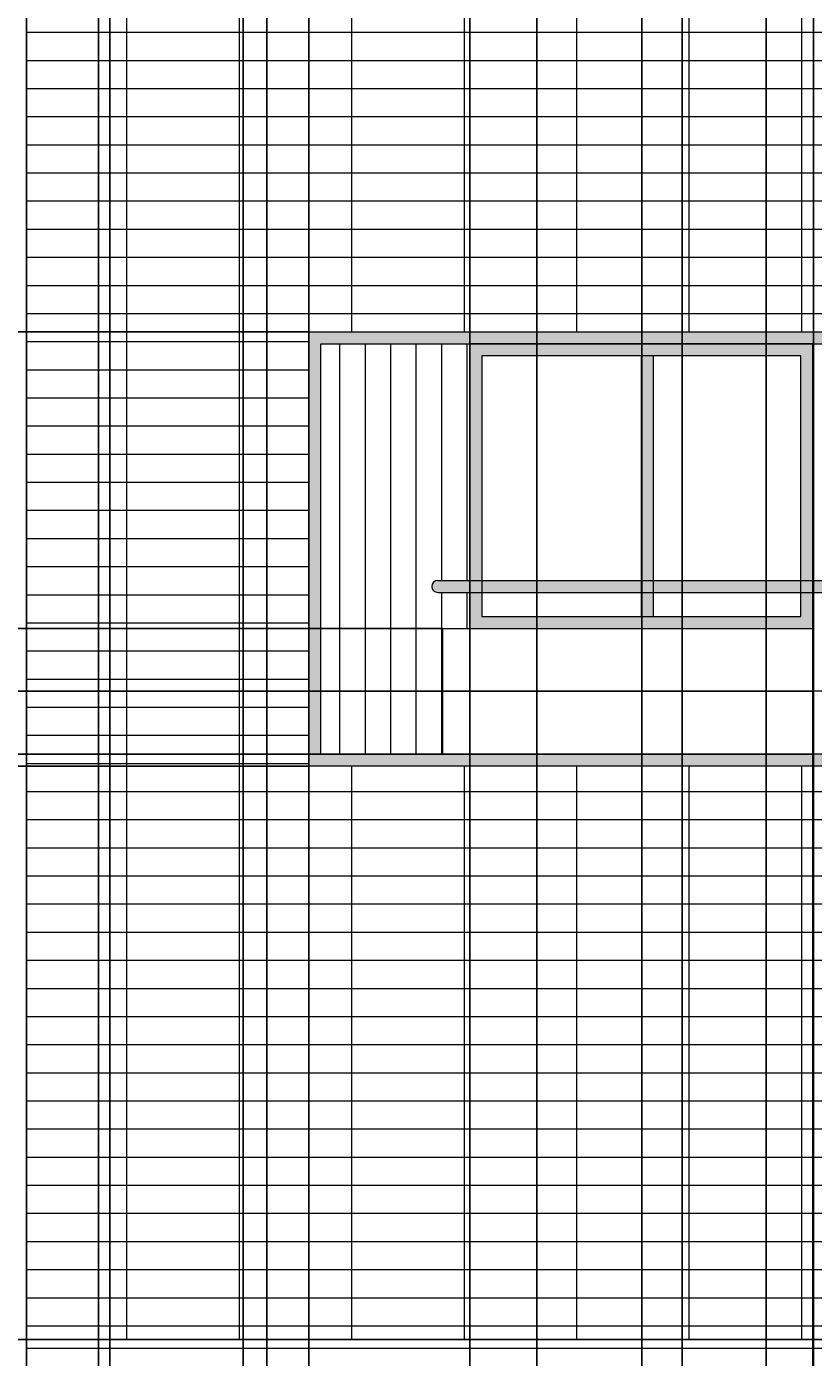
# Model space of a CAD drawing. Units: inches. Extents: x 241 to 943, y 109 to 1396.
# Tile 7 of 34: x 377 to 508, y 398 to 620. Entities that reach past the tile are written whole.
import ezdxf

# ---------------------------------------------------------------- set-up
doc = ezdxf.new("R2010")
doc.units = ezdxf.units.IN
doc.header["$MEASUREMENT"] = 0
for name, color, linetype, lineweight in [('A-ANNO-DIMS', 2, 'Continuous', 18), ('A-ELEV', 7, 'Continuous', 25), ('A-ELEV-SHAD', 9, 'Continuous', 13), ('A-GLAZ', 4, 'Continuous', 18), ('A-GLAZ-PATT', 18, 'Continuous', 13), ('A-WALL-PATT', 8, 'Continuous', 13)]:
    doc.layers.add(name, color=color, linetype=linetype, lineweight=lineweight)
doc.styles.get("Standard").update_dxf_attribs({"font": 'arial.ttf'})
doc.dimstyles.get("Standard").update_dxf_attribs({"dimtxt": 1.4375, "dimasz": 0.18, "dimexe": 0.18, "dimexo": 0.0625, "dimgap": 0.09, "dimtad": 0, "dimtih": 1, "dimtoh": 1, "dimdec": 4, "dimzin": 0, "dimdsep": 46, "dimlunit": 4, "dimtxsty": 'Standard', "dimcen": 0.09, "dimadec": 0, "dimazin": 0, "dimtfac": 1, "dimtdec": 4, "dimtofl": 0, "dimtmove": 0, "dimatfit": 3, "dimfxl": 1, "dimtolj": 1, "dimtzin": 0, "dimarcsym": 0})

# ---------------------------------------------------------------- blocks, each defined once
blk = doc.blocks.new('*D7')
at = {"layer": 'A-ANNO-DIMS', "color": 0, "lineweight": -2, "transparency": 16777216}
for p, q in [((508.24, 1336.12), (244.31, 1336.12)), ((244.49, 1335.94), (244.49, 753.25)), ((244.49, 168.92), (244.49, 751.6)), ((303.17, 168.74), (244.31, 168.74))]:
    blk.add_line(p, q, dxfattribs=at)
at = {"layer": 'A-ANNO-DIMS', "color": 0, "transparency": 16777216}
for points in [[(244.46, 1335.94), (244.52, 1335.94), (244.49, 1336.12)], [(244.46, 168.92), (244.52, 168.92), (244.49, 168.74)]]:
    blk.add_solid(points, dxfattribs=at)
at = {"layer": 'Defpoints', "color": 0, "transparency": 16777216}
for p in [(244.49, 1336.12), (508.31, 1336.12), (303.24, 168.74)]:
    blk.add_point(p, dxfattribs=at)
at = {"layer": 'A-ANNO-DIMS', "color": 0, "transparency": 16777216, "insert": (244.49, 752.43), "char_height": 1.438, "attachment_point": 5}
blk.add_mtext('\\A1;1167.4', dxfattribs=at)
blk = doc.blocks.new('*D8')
at = {"layer": 'A-ANNO-DIMS', "color": 0, "lineweight": -2, "transparency": 16777216}
for p, q in [((377.04, 396.94), (377.04, 1395.05)), ((377.22, 1394.87), (380.96, 1394.87)), ((390.71, 1394.87), (386.97, 1394.87)), ((390.89, 384.24), (390.89, 1395.05))]:
    blk.add_line(p, q, dxfattribs=at)
at = {"layer": 'A-ANNO-DIMS', "color": 0, "transparency": 16777216}
for points in [[(377.22, 1394.9), (377.22, 1394.84), (377.04, 1394.87)], [(390.71, 1394.9), (390.71, 1394.84), (390.89, 1394.87)]]:
    blk.add_solid(points, dxfattribs=at)
at = {"layer": 'Defpoints', "color": 0, "transparency": 16777216}
for p in [(390.89, 1394.87), (377.04, 396.88), (390.89, 384.18)]:
    blk.add_point(p, dxfattribs=at)
at = {"layer": 'A-ANNO-DIMS', "color": 0, "transparency": 16777216, "insert": (383.97, 1394.87), "char_height": 1.438, "attachment_point": 5}
blk.add_mtext('\\A1;13.856', dxfattribs=at)
blk = doc.blocks.new('*D9')
at = {"layer": 'A-ANNO-DIMS', "color": 0, "lineweight": -2, "transparency": 16777216}
for p, q in [((390.89, 384.24), (390.89, 1395.05)), ((391.07, 1394.87), (424.13, 1394.87)), ((461.93, 1394.87), (428.87, 1394.87)), ((462.11, 384.24), (462.11, 1395.05))]:
    blk.add_line(p, q, dxfattribs=at)
at = {"layer": 'A-ANNO-DIMS', "color": 0, "transparency": 16777216}
for points in [[(391.07, 1394.9), (391.07, 1394.84), (390.89, 1394.87)], [(461.93, 1394.9), (461.93, 1394.84), (462.11, 1394.87)]]:
    blk.add_solid(points, dxfattribs=at)
at = {"layer": 'Defpoints', "color": 0, "transparency": 16777216}
for p in [(462.11, 1394.87), (390.89, 384.18), (462.11, 384.18)]:
    blk.add_point(p, dxfattribs=at)
at = {"layer": 'A-ANNO-DIMS', "color": 0, "transparency": 16777216, "insert": (426.5, 1394.87), "char_height": 1.438, "attachment_point": 5}
blk.add_mtext('\\A1;71.21', dxfattribs=at)
blk = doc.blocks.new('*D10')
at = {"layer": 'A-ANNO-DIMS', "color": 0, "lineweight": -2, "transparency": 16777216}
for p, q in [((462.11, 384.24), (462.11, 1395.05)), ((462.29, 1394.87), (468.4, 1394.87)), ((479.42, 1394.87), (473.3, 1394.87)), ((479.6, 384.24), (479.6, 1395.05))]:
    blk.add_line(p, q, dxfattribs=at)
at = {"layer": 'A-ANNO-DIMS', "color": 0, "transparency": 16777216}
for points in [[(462.29, 1394.9), (462.29, 1394.84), (462.11, 1394.87)], [(479.42, 1394.9), (479.42, 1394.84), (479.6, 1394.87)]]:
    blk.add_solid(points, dxfattribs=at)
at = {"layer": 'Defpoints', "color": 0, "transparency": 16777216}
for p in [(479.6, 1394.87), (462.11, 384.18), (479.6, 384.18)]:
    blk.add_point(p, dxfattribs=at)
at = {"layer": 'A-ANNO-DIMS', "color": 0, "transparency": 16777216, "insert": (470.85, 1394.87), "char_height": 1.438, "attachment_point": 5}
blk.add_mtext('\\A1;17.49', dxfattribs=at)
blk = doc.blocks.new('*D11')
at = {"layer": 'A-ANNO-DIMS', "color": 0, "lineweight": -2, "transparency": 16777216}
for p, q in [((500.33, 384.24), (500.33, 1395.05)), ((500.51, 1394.87), (513.31, 1394.87)), ((530.05, 1394.87), (517.25, 1394.87)), ((530.23, 384.24), (530.23, 1395.05))]:
    blk.add_line(p, q, dxfattribs=at)
at = {"layer": 'A-ANNO-DIMS', "color": 0, "transparency": 16777216}
for points in [[(500.51, 1394.9), (500.51, 1394.84), (500.33, 1394.87)], [(530.05, 1394.9), (530.05, 1394.84), (530.23, 1394.87)]]:
    blk.add_solid(points, dxfattribs=at)
at = {"layer": 'Defpoints', "color": 0, "transparency": 16777216}
for p in [(530.23, 1394.87), (500.33, 384.18), (530.23, 384.18)]:
    blk.add_point(p, dxfattribs=at)
at = {"layer": 'A-ANNO-DIMS', "color": 0, "transparency": 16777216, "insert": (515.28, 1394.87), "char_height": 1.438, "attachment_point": 5}
blk.add_mtext('\\A1;29.9', dxfattribs=at)
blk = doc.blocks.new('*D32')
at = {"layer": 'A-ANNO-DIMS', "color": 0, "lineweight": -2, "transparency": 16777216}
for p, q in [((424.05, 568.83), (244.31, 568.83)), ((244.49, 568.65), (244.49, 533.46)), ((244.49, 496.62), (244.49, 531.81)), ((424.05, 496.44), (244.31, 496.44))]:
    blk.add_line(p, q, dxfattribs=at)
at = {"layer": 'A-ANNO-DIMS', "color": 0, "transparency": 16777216}
for points in [[(244.46, 568.65), (244.52, 568.65), (244.49, 568.83)], [(244.46, 496.62), (244.52, 496.62), (244.49, 496.44)]]:
    blk.add_solid(points, dxfattribs=at)
at = {"layer": 'Defpoints', "color": 0, "transparency": 16777216}
for p in [(244.49, 568.83), (424.11, 568.83), (424.11, 496.44)]:
    blk.add_point(p, dxfattribs=at)
at = {"layer": 'A-ANNO-DIMS', "color": 0, "transparency": 16777216, "insert": (244.49, 532.63), "char_height": 1.438, "attachment_point": 5}
blk.add_mtext('\\A1;72.39', dxfattribs=at)
blk = doc.blocks.new('*D33')
at = {"layer": 'A-ANNO-DIMS', "color": 0, "lineweight": -2, "transparency": 16777216}
for p, q in [((424.05, 628.4), (244.31, 628.4)), ((244.49, 628.22), (244.49, 599.44)), ((244.49, 569.01), (244.49, 597.79)), ((424.05, 568.83), (244.31, 568.83))]:
    blk.add_line(p, q, dxfattribs=at)
at = {"layer": 'A-ANNO-DIMS', "color": 0, "transparency": 16777216}
for points in [[(244.46, 628.22), (244.52, 628.22), (244.49, 628.4)], [(244.46, 569.01), (244.52, 569.01), (244.49, 568.83)]]:
    blk.add_solid(points, dxfattribs=at)
at = {"layer": 'Defpoints', "color": 0, "transparency": 16777216}
for p in [(244.49, 628.4), (424.11, 628.4), (424.11, 568.83)]:
    blk.add_point(p, dxfattribs=at)
at = {"layer": 'A-ANNO-DIMS', "color": 0, "transparency": 16777216, "insert": (244.49, 598.62), "char_height": 1.438, "attachment_point": 5}
blk.add_mtext('\\A1;59.57', dxfattribs=at)
blk = doc.blocks.new('*D41')
at = {"layer": 'A-ANNO-DIMS', "color": 0, "lineweight": -2, "transparency": 16777216}
for p, q in [((820.77, 400.83), (244.31, 400.83)), ((244.49, 400.65), (244.49, 317.65)), ((244.49, 233.01), (244.49, 316.01)), ((820.77, 232.83), (244.31, 232.83))]:
    blk.add_line(p, q, dxfattribs=at)
at = {"layer": 'A-ANNO-DIMS', "color": 0, "transparency": 16777216}
for points in [[(244.46, 400.65), (244.52, 400.65), (244.49, 400.83)], [(244.46, 233.01), (244.52, 233.01), (244.49, 232.83)]]:
    blk.add_solid(points, dxfattribs=at)
at = {"layer": 'Defpoints', "color": 0, "transparency": 16777216}
for p in [(244.49, 400.83), (820.84, 400.83), (820.84, 232.83)]:
    blk.add_point(p, dxfattribs=at)
at = {"layer": 'A-ANNO-DIMS', "color": 0, "transparency": 16777216, "insert": (244.49, 316.83), "char_height": 1.438, "attachment_point": 5}
blk.add_mtext('\\A1;168', dxfattribs=at)
blk = doc.blocks.new('*D61')
at = {"layer": 'A-ANNO-DIMS', "color": 0, "lineweight": -2, "transparency": 16777216}
for p, q in [((377.04, 400.89), (377.04, 1395.05)), ((377.22, 1394.87), (398.03, 1394.87)), ((423.93, 1394.87), (403.12, 1394.87)), ((424.11, 568.89), (424.11, 1395.05))]:
    blk.add_line(p, q, dxfattribs=at)
at = {"layer": 'A-ANNO-DIMS', "color": 0, "transparency": 16777216}
for points in [[(377.22, 1394.9), (377.22, 1394.84), (377.04, 1394.87)], [(423.93, 1394.9), (423.93, 1394.84), (424.11, 1394.87)]]:
    blk.add_solid(points, dxfattribs=at)
at = {"layer": 'Defpoints', "color": 0, "transparency": 16777216}
for p in [(424.11, 1394.87), (424.11, 568.83), (377.04, 400.83)]:
    blk.add_point(p, dxfattribs=at)
at = {"layer": 'A-ANNO-DIMS', "color": 0, "transparency": 16777216, "insert": (400.57, 1394.87), "char_height": 1.438, "attachment_point": 5}
blk.add_mtext('\\A1;47.07', dxfattribs=at)
blk = doc.blocks.new('*D62')
at = {"layer": 'A-ANNO-DIMS', "color": 0, "lineweight": -2, "transparency": 16777216}
for p, q in [((424.11, 568.89), (424.11, 1395.05)), ((424.29, 1394.87), (492.35, 1394.87)), ((565.02, 1394.87), (496.96, 1394.87)), ((565.2, 568.89), (565.2, 1395.05))]:
    blk.add_line(p, q, dxfattribs=at)
at = {"layer": 'A-ANNO-DIMS', "color": 0, "transparency": 16777216}
for points in [[(424.29, 1394.9), (424.29, 1394.84), (424.11, 1394.87)], [(565.02, 1394.9), (565.02, 1394.84), (565.2, 1394.87)]]:
    blk.add_solid(points, dxfattribs=at)
at = {"layer": 'Defpoints', "color": 0, "transparency": 16777216}
for p in [(565.2, 1394.87), (424.11, 568.83), (565.2, 568.83)]:
    blk.add_point(p, dxfattribs=at)
at = {"layer": 'A-ANNO-DIMS', "color": 0, "transparency": 16777216, "insert": (494.66, 1394.87), "char_height": 1.438, "attachment_point": 5}
blk.add_mtext('\\A1;141.1', dxfattribs=at)
blk = doc.blocks.new('*D79')
at = {"layer": 'A-ANNO-DIMS', "color": 0, "lineweight": -2, "transparency": 16777216}
for p, q in [((479.6, 384.24), (479.6, 1395.05)), ((479.78, 1394.87), (486.88, 1394.87)), ((500.15, 1394.87), (493.05, 1394.87)), ((500.33, 384.24), (500.33, 1395.05))]:
    blk.add_line(p, q, dxfattribs=at)
at = {"layer": 'A-ANNO-DIMS', "color": 0, "transparency": 16777216}
for points in [[(479.78, 1394.9), (479.78, 1394.84), (479.6, 1394.87)], [(500.15, 1394.9), (500.15, 1394.84), (500.33, 1394.87)]]:
    blk.add_solid(points, dxfattribs=at)
at = {"layer": 'Defpoints', "color": 0, "transparency": 16777216}
for p in [(500.33, 1394.87), (479.6, 384.18), (500.33, 384.18)]:
    blk.add_point(p, dxfattribs=at)
at = {"layer": 'A-ANNO-DIMS', "color": 0, "transparency": 16777216, "insert": (489.96, 1394.87), "char_height": 1.438, "attachment_point": 5}
blk.add_mtext('\\A1;20.736', dxfattribs=at)
blk = doc.blocks.new('*D91')
at = {"layer": 'A-ANNO-DIMS', "color": 0, "lineweight": -2, "transparency": 16777216}
for p, q in [((377.04, 1070.79), (377.04, 109.81)), ((389.04, 1070.79), (389.04, 109.81)), ((377.22, 109.99), (380.04, 109.99)), ((388.86, 109.99), (386.04, 109.99))]:
    blk.add_line(p, q, dxfattribs=at)
at = {"layer": 'A-ANNO-DIMS', "color": 0, "transparency": 16777216}
for points in [[(377.22, 110.02), (377.22, 109.96), (377.04, 109.99)], [(388.86, 110.02), (388.86, 109.96), (389.04, 109.99)]]:
    blk.add_solid(points, dxfattribs=at)
at = {"layer": 'Defpoints', "color": 0, "transparency": 16777216}
for p in [(377.04, 1070.85), (389.04, 1070.85), (389.04, 109.99)]:
    blk.add_point(p, dxfattribs=at)
at = {"layer": 'A-ANNO-DIMS', "color": 0, "transparency": 16777216, "insert": (383.04, 109.99), "char_height": 1.438, "attachment_point": 5}
blk.add_mtext('\\A1;12.004', dxfattribs=at)
blk = doc.blocks.new('*D99')
at = {"layer": 'A-ANNO-DIMS', "color": 0, "lineweight": -2, "transparency": 16777216}
for p, q in [((417.09, 181.71), (417.09, 1395.05)), ((417.27, 1394.87), (539.16, 1394.87)), ((667.21, 1394.87), (545.33, 1394.87)), ((667.39, 214.58), (667.39, 1395.05))]:
    blk.add_line(p, q, dxfattribs=at)
at = {"layer": 'A-ANNO-DIMS', "color": 0, "transparency": 16777216}
for points in [[(417.27, 1394.9), (417.27, 1394.84), (417.09, 1394.87)], [(667.21, 1394.9), (667.21, 1394.84), (667.39, 1394.87)]]:
    blk.add_solid(points, dxfattribs=at)
at = {"layer": 'Defpoints', "color": 0, "transparency": 16777216}
for p in [(667.39, 1394.87), (667.39, 214.52), (417.09, 181.65)]:
    blk.add_point(p, dxfattribs=at)
at = {"layer": 'A-ANNO-DIMS', "color": 0, "transparency": 16777216, "insert": (542.24, 1394.87), "char_height": 1.438, "attachment_point": 5}
blk.add_mtext('\\A1;250.30', dxfattribs=at)
blk = doc.blocks.new('*D126')
at = {"layer": 'A-ANNO-DIMS', "color": 0, "lineweight": -2, "transparency": 16777216}
for p, q in [((450.93, 651.27), (450.93, 109.81)), ((424.11, 628.34), (424.11, 109.81)), ((424.29, 109.99), (434.43, 109.99)), ((450.75, 109.99), (440.6, 109.99))]:
    blk.add_line(p, q, dxfattribs=at)
at = {"layer": 'A-ANNO-DIMS', "color": 0, "transparency": 16777216}
for points in [[(424.29, 110.02), (424.29, 109.96), (424.11, 109.99)], [(450.75, 110.02), (450.75, 109.96), (450.93, 109.99)]]:
    blk.add_solid(points, dxfattribs=at)
at = {"layer": 'Defpoints', "color": 0, "transparency": 16777216}
for p in [(450.93, 651.34), (424.11, 628.4), (450.93, 109.99)]:
    blk.add_point(p, dxfattribs=at)
at = {"layer": 'A-ANNO-DIMS', "color": 0, "transparency": 16777216, "insert": (437.52, 109.99), "char_height": 1.438, "attachment_point": 5}
blk.add_mtext('\\A1;26.817', dxfattribs=at)
blk = doc.blocks.new('*D127')
at = {"layer": 'A-ANNO-DIMS', "color": 0, "lineweight": -2, "transparency": 16777216}
for p, q in [((450.93, 651.27), (450.93, 109.81)), ((508.19, 630.34), (508.19, 109.81)), ((451.11, 109.99), (477.04, 109.99)), ((508.01, 109.99), (482.07, 109.99))]:
    blk.add_line(p, q, dxfattribs=at)
at = {"layer": 'A-ANNO-DIMS', "color": 0, "transparency": 16777216}
for points in [[(451.11, 110.02), (451.11, 109.96), (450.93, 109.99)], [(508.01, 110.02), (508.01, 109.96), (508.19, 109.99)]]:
    blk.add_solid(points, dxfattribs=at)
at = {"layer": 'Defpoints', "color": 0, "transparency": 16777216}
for p in [(450.93, 651.34), (508.19, 630.4), (508.19, 109.99)]:
    blk.add_point(p, dxfattribs=at)
at = {"layer": 'A-ANNO-DIMS', "color": 0, "transparency": 16777216, "insert": (479.56, 109.99), "char_height": 1.438, "attachment_point": 5}
blk.add_mtext('\\A1;57.26', dxfattribs=at)
blk = doc.blocks.new('*D128')
at = {"layer": 'A-ANNO-DIMS', "color": 0, "lineweight": -2, "transparency": 16777216}
for p, q in [((534.18, 651.27), (534.18, 109.81)), ((508.19, 630.34), (508.19, 109.81)), ((508.37, 109.99), (518.1, 109.99)), ((534, 109.99), (524.27, 109.99))]:
    blk.add_line(p, q, dxfattribs=at)
at = {"layer": 'A-ANNO-DIMS', "color": 0, "transparency": 16777216}
for points in [[(508.37, 110.02), (508.37, 109.96), (508.19, 109.99)], [(534, 110.02), (534, 109.96), (534.18, 109.99)]]:
    blk.add_solid(points, dxfattribs=at)
at = {"layer": 'Defpoints', "color": 0, "transparency": 16777216}
for p in [(534.18, 651.34), (508.19, 630.4), (534.18, 109.99)]:
    blk.add_point(p, dxfattribs=at)
at = {"layer": 'A-ANNO-DIMS', "color": 0, "transparency": 16777216, "insert": (521.18, 109.99), "char_height": 1.438, "attachment_point": 5}
blk.add_mtext('\\A1;25.987', dxfattribs=at)
blk = doc.blocks.new('*D136')
at = {"layer": 'A-ANNO-DIMS', "color": 0, "lineweight": -2, "transparency": 16777216}
for p, q in [((450.93, 519.31), (450.93, 109.81)), ((424.11, 496.38), (424.11, 109.81)), ((424.29, 109.99), (434.43, 109.99)), ((450.75, 109.99), (440.6, 109.99))]:
    blk.add_line(p, q, dxfattribs=at)
at = {"layer": 'A-ANNO-DIMS', "color": 0, "transparency": 16777216}
for points in [[(424.29, 110.02), (424.29, 109.96), (424.11, 109.99)], [(450.75, 110.02), (450.75, 109.96), (450.93, 109.99)]]:
    blk.add_solid(points, dxfattribs=at)
at = {"layer": 'Defpoints', "color": 0, "transparency": 16777216}
for p in [(450.93, 519.38), (424.11, 496.44), (450.93, 109.99)]:
    blk.add_point(p, dxfattribs=at)
at = {"layer": 'A-ANNO-DIMS', "color": 0, "transparency": 16777216, "insert": (437.52, 109.99), "char_height": 1.438, "attachment_point": 5}
blk.add_mtext('\\A1;26.817', dxfattribs=at)
blk = doc.blocks.new('*D137')
at = {"layer": 'A-ANNO-DIMS', "color": 0, "lineweight": -2, "transparency": 16777216}
for p, q in [((450.93, 519.31), (450.93, 109.81)), ((508.08, 508.84), (508.08, 109.81)), ((451.11, 109.99), (476.98, 109.99)), ((507.9, 109.99), (482.02, 109.99))]:
    blk.add_line(p, q, dxfattribs=at)
at = {"layer": 'A-ANNO-DIMS', "color": 0, "transparency": 16777216}
for points in [[(451.11, 110.02), (451.11, 109.96), (450.93, 109.99)], [(507.9, 110.02), (507.9, 109.96), (508.08, 109.99)]]:
    blk.add_solid(points, dxfattribs=at)
at = {"layer": 'Defpoints', "color": 0, "transparency": 16777216}
for p in [(450.93, 519.38), (508.08, 508.91), (508.08, 109.99)]:
    blk.add_point(p, dxfattribs=at)
at = {"layer": 'A-ANNO-DIMS', "color": 0, "transparency": 16777216, "insert": (479.5, 109.99), "char_height": 1.438, "attachment_point": 5}
blk.add_mtext('\\A1;57.15', dxfattribs=at)
blk = doc.blocks.new('*D138')
at = {"layer": 'A-ANNO-DIMS', "color": 0, "lineweight": -2, "transparency": 16777216}
for p, q in [((508.08, 508.84), (508.08, 109.81)), ((534.18, 508.84), (534.18, 109.81)), ((508.26, 109.99), (518.6, 109.99)), ((534, 109.99), (523.65, 109.99))]:
    blk.add_line(p, q, dxfattribs=at)
at = {"layer": 'A-ANNO-DIMS', "color": 0, "transparency": 16777216}
for points in [[(508.26, 110.02), (508.26, 109.96), (508.08, 109.99)], [(534, 110.02), (534, 109.96), (534.18, 109.99)]]:
    blk.add_solid(points, dxfattribs=at)
at = {"layer": 'Defpoints', "color": 0, "transparency": 16777216}
for p in [(508.08, 508.91), (534.18, 508.91), (534.18, 109.99)]:
    blk.add_point(p, dxfattribs=at)
at = {"layer": 'A-ANNO-DIMS', "color": 0, "transparency": 16777216, "insert": (521.13, 109.99), "char_height": 1.438, "attachment_point": 5}
blk.add_mtext('\\A1;26.10', dxfattribs=at)
blk = doc.blocks.new('*D140')
at = {"layer": 'A-ANNO-DIMS', "color": 0, "lineweight": -2, "transparency": 16777216}
for p, q in [((446.37, 519.38), (244.31, 519.38)), ((244.49, 519.2), (244.49, 509.73)), ((244.49, 498.62), (244.49, 508.08)), ((446.37, 498.44), (244.31, 498.44))]:
    blk.add_line(p, q, dxfattribs=at)
at = {"layer": 'A-ANNO-DIMS', "color": 0, "transparency": 16777216}
for points in [[(244.46, 519.2), (244.52, 519.2), (244.49, 519.38)], [(244.46, 498.62), (244.52, 498.62), (244.49, 498.44)]]:
    blk.add_solid(points, dxfattribs=at)
at = {"layer": 'Defpoints', "color": 0, "transparency": 16777216}
for p in [(244.49, 519.38), (446.43, 519.38), (446.43, 498.44)]:
    blk.add_point(p, dxfattribs=at)
at = {"layer": 'A-ANNO-DIMS', "color": 0, "transparency": 16777216, "insert": (244.49, 508.91), "char_height": 1.438, "attachment_point": 5}
blk.add_mtext('\\A1;20.936', dxfattribs=at)
blk = doc.blocks.new('*D141')
at = {"layer": 'A-ANNO-DIMS', "color": 0, "lineweight": -2, "transparency": 16777216}
for p, q in [((508.13, 508.91), (244.31, 508.91)), ((244.49, 508.73), (244.49, 504.5)), ((244.49, 498.62), (244.49, 502.85)), ((508.13, 498.44), (244.31, 498.44))]:
    blk.add_line(p, q, dxfattribs=at)
at = {"layer": 'A-ANNO-DIMS', "color": 0, "transparency": 16777216}
for points in [[(244.46, 508.73), (244.52, 508.73), (244.49, 508.91)], [(244.46, 498.62), (244.52, 498.62), (244.49, 498.44)]]:
    blk.add_solid(points, dxfattribs=at)
at = {"layer": 'Defpoints', "color": 0, "transparency": 16777216}
for p in [(244.49, 508.91), (508.19, 508.91), (508.19, 498.44)]:
    blk.add_point(p, dxfattribs=at)
at = {"layer": 'A-ANNO-DIMS', "color": 0, "transparency": 16777216, "insert": (244.49, 503.67), "char_height": 1.438, "attachment_point": 5}
blk.add_mtext('\\A1;10.468', dxfattribs=at)
blk = doc.blocks.new('*D147')
at = {"layer": 'A-ANNO-DIMS', "color": 0, "lineweight": -2, "transparency": 16777216}
for p, q in [((389.04, 734.79), (389.04, 109.81)), ((413.12, 734.79), (413.12, 109.81)), ((389.22, 109.99), (398, 109.99)), ((412.94, 109.99), (404.17, 109.99))]:
    blk.add_line(p, q, dxfattribs=at)
at = {"layer": 'A-ANNO-DIMS', "color": 0, "transparency": 16777216}
for points in [[(389.22, 110.02), (389.22, 109.96), (389.04, 109.99)], [(412.94, 110.02), (412.94, 109.96), (413.12, 109.99)]]:
    blk.add_solid(points, dxfattribs=at)
at = {"layer": 'Defpoints', "color": 0, "transparency": 16777216}
for p in [(389.04, 734.85), (413.12, 734.85), (413.12, 109.99)]:
    blk.add_point(p, dxfattribs=at)
at = {"layer": 'A-ANNO-DIMS', "color": 0, "transparency": 16777216, "insert": (401.08, 109.99), "char_height": 1.438, "attachment_point": 5}
blk.add_mtext('\\A1;24.076', dxfattribs=at)
blk = doc.blocks.new('*D148')
at = {"layer": 'A-ANNO-DIMS', "color": 0, "lineweight": -2, "transparency": 16777216}
for p, q in [((413.12, 734.79), (413.12, 109.81)), ((486.34, 734.79), (486.34, 109.81)), ((413.3, 109.99), (447.23, 109.99)), ((486.16, 109.99), (452.23, 109.99))]:
    blk.add_line(p, q, dxfattribs=at)
at = {"layer": 'A-ANNO-DIMS', "color": 0, "transparency": 16777216}
for points in [[(413.3, 110.02), (413.3, 109.96), (413.12, 109.99)], [(486.16, 110.02), (486.16, 109.96), (486.34, 109.99)]]:
    blk.add_solid(points, dxfattribs=at)
at = {"layer": 'Defpoints', "color": 0, "transparency": 16777216}
for p in [(413.12, 734.85), (486.34, 734.85), (486.34, 109.99)]:
    blk.add_point(p, dxfattribs=at)
at = {"layer": 'A-ANNO-DIMS', "color": 0, "transparency": 16777216, "insert": (449.73, 109.99), "char_height": 1.438, "attachment_point": 5}
blk.add_mtext('\\A1;73.22', dxfattribs=at)

msp = doc.modelspace()

# ---------------------------------------------------------------- hatches: boundary and pattern name
at = {"layer": 'A-ELEV-SHAD'}
h = msp.add_hatch(color=256, dxfattribs=at)
h.dxf.hatch_style = 1
h.paths.add_polyline_path([(537.4269, 566.8295), (534.1778, 566.8295), (534.1778, 527.3816), (537.4269, 527.3816)])
h.paths.add_polyline_path([(508.0803, 566.8295), (450.9259, 566.8295), (450.9259, 527.3816), (452.9259, 527.3816), (452.9259, 564.8295), (506.0803, 564.8295), (506.0803, 527.3816), (508.0803, 527.3816)])
h.paths.add_polyline_path([(481.5031, 564.8295), (479.5031, 564.8295), (479.5031, 527.3816), (481.5031, 527.3816)], flags=17)
h.paths.add_polyline_path([(481.5031, 525.3816), (479.5031, 525.3816), (479.5031, 521.3754), (481.5031, 521.3754)], flags=17)
h.paths.add_polyline_path([(508.0803, 525.3816), (506.0803, 525.3816), (506.0803, 521.3754), (452.9259, 521.3754), (452.9259, 525.3816), (450.9259, 525.3816), (450.9259, 519.3754), (508.0803, 519.3754)])
h.paths.add_polyline_path([(537.4269, 525.3816), (534.1778, 525.3816), (534.1778, 508.9074), (537.4269, 508.9074)])
h.paths.add_polyline_path([(749.6328, 702.7912), (617.7594, 702.7912), (617.7594, 700.7912), (747.6328, 700.7912), (747.6328, 628.4013), (617.7594, 628.4013), (617.7594, 626.4013), (749.6328, 626.4013)])
h.paths.add_polyline_path([(652.0129, 700.7912), (650.0129, 700.7912), (650.0129, 628.4013), (652.0129, 628.4013)], flags=17)
h.paths.add_polyline_path([(678.8698, 700.7912), (676.8698, 700.7912), (676.8698, 628.4013), (678.8698, 628.4013)], flags=17)
h.paths.add_polyline_path([(712.0171, 700.7912), (710.0171, 700.7912), (710.0171, 628.4013), (712.0171, 628.4013)], flags=17)
h.paths.add_polyline_path([(710.0171, 675.7856), (678.8698, 675.7856), (678.8698, 673.7856), (710.0171, 673.7856)], flags=17)
h.paths.add_polyline_path([(537.4269, 698.7912), (534.1778, 698.7912), (534.1778, 659.3434), (537.4269, 659.3434)], flags=0)
h.paths.add_polyline_path([(592.9542, 700.7912), (424.1086, 700.7912), (424.1086, 628.4013), (592.9542, 628.4013)])
h.paths.add_polyline_path([(590.8792, 698.7912), (590.8792, 630.4013), (426.1086, 630.4013), (426.1086, 698.7912)], flags=16)
h.paths.add_polyline_path([(563.2023, 698.7912), (563.2023, 659.3434), (563.9297, 659.3434), (563.9297, 651.3371), (508.1906, 651.3371), (508.0803, 651.3371), (450.9259, 651.3371), (428.0291, 651.3371), (428.0291, 698.7912), (451.9767, 698.7912), (508.0803, 698.7912), (537.4269, 698.7912)], flags=0)
h.paths.add_polyline_path([(506.0803, 696.7912), (506.0803, 653.3371), (452.9259, 653.3371), (452.9259, 657.3434), (445.5808, 657.3434, -1), (445.5808, 659.3434), (452.9259, 659.3434), (452.9259, 696.7912)], flags=0)
h.paths.add_polyline_path([(563.9297, 698.7912), (563.2023, 698.7912), (563.2023, 659.3434), (563.9297, 659.3434)], flags=0)
h = msp.add_hatch(color=256, dxfattribs=at)
h.dxf.hatch_style = 1
h.paths.add_polyline_path([(748.3325, 566.8295), (746.3325, 566.8295), (746.3325, 498.4395), (748.3325, 498.4395)])
h.paths.add_polyline_path([(746.3325, 524.3723), (691.794, 524.3723), (691.794, 522.3723), (746.3325, 522.3723)])
h.paths.add_polyline_path([(691.794, 566.8295), (689.794, 566.8295), (689.794, 498.4395), (691.794, 498.4395)])
h.paths.add_polyline_path([(790.691, 542.7994), (748.3325, 542.7994), (748.3325, 540.7994), (790.691, 540.7994)])
h.paths.add_polyline_path([(500.3323, 384.1784), (479.596, 384.1784), (479.596, 289.6933), (500.3323, 289.6933)])
h.paths.add_polyline_path([(481.596, 291.6933), (481.596, 382.1784), (498.3323, 382.1784), (498.3323, 291.6933)], flags=16)
h.paths.add_polyline_path([(462.1074, 384.1784), (390.895, 384.1784), (390.895, 289.6933), (462.1074, 289.6933)])
h.paths.add_polyline_path([(392.895, 291.6933), (392.895, 382.1784), (460.1074, 382.1784), (460.1074, 291.6933)], flags=16)
h.paths.add_polyline_path([(794.0275, 289.9984), (667.3935, 289.9984), (667.3935, 214.5189), (794.0275, 214.5189)])
h.paths.add_polyline_path([(792.0275, 287.9984), (792.0275, 216.5189), (669.3935, 216.5189), (669.3935, 287.9984)], flags=16)
h.paths.add_polyline_path([(508.0803, 525.3816), (506.0803, 525.3816), (506.0803, 521.3754), (452.9259, 521.3754), (452.9259, 525.3816), (450.9259, 525.3816), (450.9259, 519.3754), (508.0803, 519.3754)], flags=0)
h.paths.add_polyline_path([(508.0803, 566.8295), (450.9259, 566.8295), (450.9259, 527.3816), (452.9259, 527.3816), (452.9259, 564.8295), (506.0803, 564.8295), (506.0803, 527.3816), (508.0803, 527.3816)], flags=0)
h.paths.add_polyline_path([(537.4269, 566.8295), (534.1778, 566.8295), (534.1778, 527.3816), (537.4269, 527.3816)], flags=0)
h.paths.add_polyline_path([(537.4269, 525.3816), (534.1778, 525.3816), (534.1778, 508.9074), (537.4269, 508.9074)], flags=0)
h.paths.add_polyline_path([(565.2023, 568.8295), (424.1086, 568.8295), (424.1086, 496.4395), (565.2023, 496.4395)])
h.paths.add_polyline_path([(563.2023, 508.9074), (563.2023, 498.4395), (426.1086, 498.4395), (426.1086, 566.8295), (563.2023, 566.8295)], flags=16)
h.paths.add_polyline_path([(508.0803, 508.9074), (508.0803, 519.3754), (450.9259, 519.3754), (450.9259, 525.3816), (445.5808, 525.3816, -1), (445.5808, 527.3816), (450.9259, 527.3816), (450.9259, 566.8295), (508.0803, 566.8295), (537.4269, 566.8295), (537.4269, 508.9074)], flags=0)
h.paths.add_polyline_path([(506.0803, 521.3754), (452.9259, 521.3754), (452.9259, 564.8295), (506.0803, 564.8295)], flags=0)
at = {"layer": 'A-GLAZ-PATT'}
h = msp.add_hatch(dxfattribs=at)
h.set_pattern_fill('ANSI31', color=256, scale=34, angle=45)
h.paths.add_polyline_path([(486.3418, 786.9154), (413.1187, 786.9154), (413.1187, 761.2284), (486.3418, 761.2284)])
h.paths.add_polyline_path([(486.3418, 954.9154), (413.1187, 954.9154), (413.1187, 929.2284), (486.3418, 929.2284)])
h.paths.add_polyline_path([(462.1074, 289.6933), (390.895, 289.6933), (390.895, 277.4626), (390.895, 274.3507), (462.1074, 274.3507), (462.1074, 277.4626)])
h.paths.add_polyline_path([(500.3323, 289.6933), (479.596, 289.6933), (479.596, 274.3507), (500.3323, 274.3507)])
h.paths.add_polyline_path([(450.9259, 566.8295), (426.1086, 566.8295), (426.1086, 498.4395), (446.4348, 498.4395), (446.4348, 519.3754), (450.9259, 519.3754), (450.9259, 525.3816), (445.5808, 525.3816, -1), (445.5808, 527.3816), (450.9259, 527.3816)])
h.paths.add_polyline_path([(563.2023, 508.9074), (534.1778, 508.9074), (508.1906, 508.9074), (508.1906, 498.4395), (563.2023, 498.4395)])
h.paths.add_polyline_path([(747.6328, 700.7912), (712.0171, 700.7912), (712.0171, 628.4013), (747.6328, 628.4013)])
h.paths.add_polyline_path([(446.4348, 643.7483), (426.1086, 643.7483), (426.1086, 630.4013), (446.4348, 630.4013)])
h.paths.add_polyline_path([(564.8076, 841.5382), (553.5166, 841.5382), (508.3064, 841.5382), (508.3064, 782.5808), (564.8076, 782.5808)])
h.paths.add_polyline_path([(564.8076, 780.5808), (508.3064, 780.5808), (508.3064, 773.4916), (564.8076, 773.4916)])
h.paths.add_polyline_path([(792.691, 762.5799), (759.6248, 762.5799), (759.6248, 736.9235), (759.6248, 734.8538), (792.691, 734.8538)])
h.paths.add_polyline_path([(564.8076, 1009.5382), (553.5166, 1009.5382), (508.3064, 1009.5382), (508.3064, 950.5808), (562.3033, 950.5808, -1), (562.3033, 948.5808), (508.3064, 948.5808), (508.3064, 941.4916), (564.8076, 941.4916)])
h.paths.add_polyline_path([(486.3418, 1122.9154), (413.1187, 1122.9154), (413.1187, 1097.2284), (486.3418, 1097.2284)])
h = msp.add_hatch(color=256, dxfattribs=at)
h.dxf.hatch_style = 1
h.paths.add_polyline_path([(396.3125, 1118.5808), (390.5597, 1118.5808), (388.0428, 1118.5808, 1), (388.0428, 1116.5808), (390.5597, 1116.5808), (396.3125, 1116.5808)])
h.paths.add_polyline_path([(398.3125, 1118.5808), (396.3125, 1118.5808), (396.3125, 1116.5808), (398.3125, 1116.5808)])
h.paths.add_polyline_path([(413.1187, 1118.5808), (398.3125, 1118.5808), (398.3125, 1116.5808), (413.1187, 1116.5808)])
h.paths.add_polyline_path([(506.3064, 1118.5808), (486.3418, 1118.5808), (486.3418, 1116.5808), (506.3064, 1116.5808)])
h.paths.add_polyline_path([(506.8039, 1118.5808), (506.3064, 1118.5808), (506.3064, 1116.5808), (506.8039, 1116.5808, 1)])
h.paths.add_polyline_path([(396.3125, 950.5808), (390.5597, 950.5808), (388.0428, 950.5808, 1), (388.0428, 948.5808), (390.5597, 948.5808), (396.3125, 948.5808)])
h.paths.add_polyline_path([(398.3125, 950.5808), (396.3125, 950.5808), (396.3125, 948.5808), (398.3125, 948.5808)])
h.paths.add_polyline_path([(413.1187, 950.5808), (398.3125, 950.5808), (398.3125, 948.5808), (413.1187, 948.5808)])
h.paths.add_polyline_path([(506.3064, 950.5808), (486.3418, 950.5808), (486.3418, 948.5808), (506.3064, 948.5808)])
h.paths.add_polyline_path([(508.3064, 950.5808), (506.3064, 950.5808), (506.3064, 948.5808), (508.3064, 948.5808)])
h.paths.add_polyline_path([(562.3033, 950.5808), (508.3064, 950.5808), (508.3064, 948.5808), (562.3033, 948.5808, 1)])
h.paths.add_polyline_path([(396.3125, 782.5808), (390.5597, 782.5808), (388.0428, 782.5808, 1), (388.0428, 780.5808), (390.5597, 780.5808), (396.3125, 780.5808)])
h.paths.add_polyline_path([(398.3125, 782.5808), (396.3125, 782.5808), (396.3125, 780.5808), (398.3125, 780.5808)])
h.paths.add_polyline_path([(413.1187, 782.5808), (398.3125, 782.5808), (398.3125, 780.5808), (413.1187, 780.5808)])
h.paths.add_polyline_path([(506.3064, 782.5808), (486.3418, 782.5808), (486.3418, 780.5808), (506.3064, 780.5808)])
h.paths.add_polyline_path([(508.3064, 782.5808), (506.3064, 782.5808), (506.3064, 780.5808), (508.3064, 780.5808)])
h.paths.add_polyline_path([(564.8076, 782.5808), (508.3064, 782.5808), (508.3064, 780.5808), (564.8076, 780.5808)])
h.paths.add_polyline_path([(605.9087, 782.5808), (564.8076, 782.5808), (564.8076, 780.5808), (605.9087, 780.5808, 1)])
h.paths.add_polyline_path([(450.9259, 659.3434), (445.5808, 659.3434, 1), (445.5808, 657.3434), (450.9259, 657.3434)])
h.paths.add_polyline_path([(452.9259, 659.3434), (450.9259, 659.3434), (450.9259, 657.3434), (452.9259, 657.3434)])
h.paths.add_polyline_path([(506.0803, 659.3434), (452.9259, 659.3434), (452.9259, 657.3434), (506.0803, 657.3434)])
h.paths.add_polyline_path([(508.0803, 659.3434), (506.0803, 659.3434), (506.0803, 657.3434), (508.0803, 657.3434)])
h.paths.add_polyline_path([(563.2023, 659.3434), (537.4269, 659.3434), (537.4269, 657.3434), (563.2023, 657.3434)])
h.paths.add_polyline_path([(590.8792, 659.3434), (563.9297, 659.3434), (563.9297, 657.3434), (590.8792, 657.3434)])
h.paths.add_polyline_path([(563.9297, 659.3434), (563.2023, 659.3434), (563.2023, 657.3434), (563.9297, 657.3434)])
h.paths.add_polyline_path([(537.4269, 659.3434), (534.1778, 659.3434), (534.1778, 657.3434), (537.4269, 657.3434)])
h.paths.add_polyline_path([(534.1778, 659.3434), (508.0803, 659.3434), (508.0803, 657.3434), (534.1778, 657.3434)])
h.paths.add_polyline_path([(450.9259, 527.3816), (445.5808, 527.3816, 1), (445.5808, 525.3816), (450.9259, 525.3816)])
h.paths.add_polyline_path([(452.9259, 527.3816), (450.9259, 527.3816), (450.9259, 525.3816), (452.9259, 525.3816)])
h.paths.add_polyline_path([(479.5031, 527.3816), (452.9259, 527.3816), (452.9259, 525.3816), (479.5031, 525.3816)])
h.paths.add_polyline_path([(481.5031, 527.3816), (479.5031, 527.3816), (479.5031, 525.3816), (481.5031, 525.3816)])
h.paths.add_polyline_path([(506.0803, 527.3816), (481.5031, 527.3816), (481.5031, 525.3816), (506.0803, 525.3816)])
h.paths.add_polyline_path([(508.0803, 527.3816), (506.0803, 527.3816), (506.0803, 525.3816), (508.0803, 525.3816)])
h.paths.add_polyline_path([(563.2023, 527.3816), (508.0803, 527.3816), (508.0803, 525.3816), (563.2023, 525.3816)])
at = {"layer": 'A-WALL-PATT'}
h = msp.add_hatch(dxfattribs=at)
h.set_pattern_fill('GRATE', color=256, scale=150)
h.paths.add_polyline_path([(747.7579, 1238.8538), (747.7579, 1275.9142), (747.7579, 1336.1154), (508.3064, 1336.1154), (508.3064, 1275.9142), (508.3064, 1238.8538), (508.3064, 1177.5382), (508.3064, 1109.4916), (508.3064, 1070.8538), (553.5166, 1070.8538), (749.6328, 1070.8538)])
h.paths.add_polyline_path([(533.952, 1108.1686), (533.952, 1177.7336), (533.952, 1303.0286), (724.819, 1303.0286), (724.819, 1108.1686)], flags=16)
h.paths.add_polyline_path([(535.952, 1110.1686), (535.952, 1175.7336), (722.819, 1175.7336), (722.819, 1110.1686)], flags=0)
h.paths.add_polyline_path([(643.4534, 1134.0739), (622.521, 1134.0739), (622.521, 1136.0739), (643.4534, 1136.0739)], flags=0)
h.paths.add_polyline_path([(617.7594, 568.8295), (617.7594, 734.8538), (377.0391, 734.8538), (377.0391, 566.8538), (377.0391, 400.8295), (417.0913, 400.8295), (618.9643, 400.8295)])
h.paths.add_polyline_path([(424.1086, 496.4395), (424.1086, 568.8295), (565.2023, 568.8295), (565.2023, 496.4395)], flags=16)
h.paths.add_polyline_path([(426.1086, 498.4395), (426.1086, 566.8295), (563.2023, 566.8295), (563.2023, 508.9074), (563.2023, 498.4395)], flags=0)
h.paths.add_polyline_path([(508.0803, 508.9074), (508.0803, 519.3754), (450.9259, 519.3754), (450.9259, 525.3816), (445.5808, 525.3816, -1), (445.5808, 527.3816), (450.9259, 527.3816), (450.9259, 566.8295), (508.0803, 566.8295), (537.4269, 566.8295), (537.4269, 508.9074)], flags=0)
h.paths.add_polyline_path([(506.0803, 521.3754), (452.9259, 521.3754), (452.9259, 564.8295), (506.0803, 564.8295)], flags=0)
h.paths.add_polyline_path([(424.1086, 628.4013), (424.1086, 700.7912), (592.9542, 700.7912), (592.9542, 628.4013)], flags=16)
h.paths.add_polyline_path([(426.1086, 630.4013), (426.1086, 698.7912), (590.8792, 698.7912), (590.8792, 630.4013)], flags=0)
h.paths.add_polyline_path([(508.1906, 651.3371), (508.0803, 651.3371), (450.9259, 651.3371), (428.0291, 651.3371), (428.0291, 698.7912), (451.9767, 698.7912), (508.0803, 698.7912), (537.4269, 698.7912), (563.2023, 698.7912), (563.2023, 659.3434), (563.9297, 659.3434), (563.9297, 651.3371)], flags=0)
h.paths.add_polyline_path([(506.0803, 653.3371), (452.9259, 653.3371), (452.9259, 657.3434), (445.5808, 657.3434, -1), (445.5808, 659.3434), (452.9259, 659.3434), (452.9259, 696.7912), (506.0803, 696.7912)], flags=0)
h = msp.add_hatch(dxfattribs=at)
h.set_pattern_fill('ANSI32', color=256, scale=71, angle=135)
h.paths.add_polyline_path([(820.8374, 568.8295), (792.691, 568.8295), (792.691, 496.4395), (651.5974, 496.4395), (651.5974, 568.8295), (617.7594, 568.8295), (618.9643, 400.8295), (417.0913, 400.8295), (377.0391, 400.8295), (377.0391, 398.8538), (377.0391, 396.8782), (377.0391, 228.8782), (377.0391, 177.6977), (416.5078, 181.5724), (417.0913, 181.649), (530.2303, 196.5065), (530.2303, 384.1784), (650.907, 384.1784), (651.7861, 212.4693), (667.3935, 214.5189), (667.3935, 289.9984), (794.0275, 289.9984), (794.0275, 232.8295), (820.8374, 232.8295), (820.8374, 400.8295)])
h.paths.add_polyline_path([(500.3323, 384.1784), (500.3323, 289.6933), (500.3323, 274.3507), (479.596, 274.3507), (479.596, 289.6933), (479.596, 384.1784)], flags=16)
h.paths.add_polyline_path([(498.3323, 382.1784), (498.3323, 291.6933), (481.596, 291.6933), (481.596, 382.1784)], flags=0)
h.paths.add_polyline_path([(462.1074, 384.1784), (462.1074, 289.6933), (462.1074, 277.4626), (462.1074, 274.3507), (390.895, 274.3507), (390.895, 277.4626), (390.895, 289.6933), (390.895, 384.1784)], flags=16)
h.paths.add_polyline_path([(460.1074, 382.1784), (460.1074, 291.6933), (392.895, 291.6933), (392.895, 382.1784)], flags=0)
h.paths.add_polyline_path([(595.3136, 372.9401), (641.6196, 372.9401), (641.6196, 246.4081), (651.6121, 246.4593), (650.907, 384.1784), (530.2303, 384.1784), (530.2303, 245.8378), (595.3136, 246.1711)], flags=17)

# ---------------------------------------------------------------- linework, layer by layer
at = {"layer": 'A-ELEV'}
for p, q in [((377.0391, 566.8538), (377.0391, 734.8538)), ((377.0391, 398.8538), (377.0391, 566.8538)), ((417.0913, 400.8295), (377.0391, 400.8295)), ((377.0391, 396.8782), (377.0391, 400.8295)), ((417.0913, 400.8295), (618.9643, 400.8295))]:
    msp.add_line(p, q, dxfattribs=at)
at = {"layer": 'A-GLAZ'}
for p, q in [((479.5031, 564.8295), (479.5031, 521.3754)), ((481.5031, 564.8295), (481.5031, 521.3754)), ((445.5808, 527.3816), (563.2023, 527.3816)), ((445.5808, 525.3816), (563.2023, 525.3816)), ((446.4348, 498.4395), (446.4348, 519.3754)), ((446.4348, 519.3754), (508.1906, 519.3754))]:
    msp.add_line(p, q, dxfattribs=at)
for points in [[(424.1086, 568.8295), (565.2023, 568.8295), (565.2023, 496.4395), (424.1086, 496.4395)], [(426.1086, 566.8295), (563.2023, 566.8295), (563.2023, 498.4395), (426.1086, 498.4395)], [(450.9259, 519.3754), (508.0803, 519.3754), (508.0803, 566.8295), (450.9259, 566.8295)], [(508.0803, 566.8295), (537.4269, 566.8295), (537.4269, 508.9074), (508.0803, 508.9074)], [(452.9259, 521.3754), (506.0803, 521.3754), (506.0803, 564.8295), (452.9259, 564.8295)]]:
    msp.add_lwpolyline(points, close=True, dxfattribs=at)
msp.add_arc((445.5808, 526.3816), 1, 90, 270, dxfattribs=at)

# ---------------------------------------------------------------- dimensions: what is measured, and where the dimension line sits
at = {"layer": 'A-ANNO-DIMS'}
for base, p1, p2, override, picture, middle in [((390.895, 1394.8654), (377.0391, 396.8782), (390.895, 384.1784), {"dimdec": 3, "dimlfac": 1, "dimrnd": 0, "dimzin": 0, "dimdsep": 46, "dimlunit": 2}, '*D8', (383.9671, 1394.8654)), ((424.1086, 1394.8654), (377.0391, 400.8295), (424.1086, 568.8295), {"dimdec": 2, "dimlfac": 1, "dimrnd": 0, "dimzin": 0, "dimdsep": 46, "dimlunit": 2}, '*D61', (400.5739, 1394.8654)), ((462.1074, 1394.8654), (390.895, 384.1784), (462.1074, 384.1784), {"dimdec": 2, "dimlfac": 1, "dimrnd": 0, "dimzin": 0, "dimdsep": 46, "dimlunit": 2}, '*D9', (426.5012, 1394.8654)), ((667.3935, 1394.8654), (417.0913, 181.649), (667.3935, 214.5189), {"dimdec": 2, "dimlfac": 1, "dimrnd": 0, "dimzin": 0, "dimdsep": 46, "dimlunit": 2}, '*D99', (542.2424, 1394.8654)), ((565.2023, 1394.8654), (424.1086, 568.8295), (565.2023, 568.8295), {"dimdec": 1, "dimlfac": 1, "dimrnd": 0, "dimzin": 0, "dimdsep": 46, "dimlunit": 2}, '*D62', (494.6554, 1394.8654)), ((479.596, 1394.8654), (462.1074, 384.1784), (479.596, 384.1784), {"dimdec": 2, "dimlfac": 1, "dimrnd": 0, "dimzin": 0, "dimdsep": 46, "dimlunit": 2}, '*D10', (470.8517, 1394.8654)), ((500.3323, 1394.8654), (479.596, 384.1784), (500.3323, 384.1784), {"dimdec": 3, "dimlfac": 1, "dimrnd": 0, "dimzin": 0, "dimdsep": 46, "dimlunit": 2}, '*D79', (489.9641, 1394.8654)), ((530.2303, 1394.8654), (500.3323, 384.1784), (530.2303, 384.1784), {"dimdec": 1, "dimlfac": 1, "dimrnd": 0, "dimzin": 0, "dimdsep": 46, "dimlunit": 2}, '*D11', (515.2813, 1394.8654)), ((389.0429, 109.9907), (377.0391, 1070.8538), (389.0429, 1070.8538), {"dimdec": 3, "dimlfac": 1, "dimrnd": 0, "dimzin": 0, "dimdsep": 46, "dimlunit": 2}, '*D91', (383.041, 109.9907)), ((413.1187, 109.9907), (389.0429, 734.8538), (413.1187, 734.8538), {"dimdec": 3, "dimlfac": 1, "dimrnd": 0, "dimzin": 0, "dimdsep": 46, "dimlunit": 2}, '*D147', (401.0808, 109.9907)), ((486.3418, 109.9907), (413.1187, 734.8538), (486.3418, 734.8538), {"dimdec": 2, "dimlfac": 1, "dimrnd": 0, "dimzin": 0, "dimdsep": 46, "dimlunit": 2}, '*D148', (449.7303, 109.9907)), ((450.9259, 109.9907), (424.1086, 628.4013), (450.9259, 651.3371), {"dimdec": 3, "dimlfac": 1, "dimrnd": 0, "dimzin": 0, "dimdsep": 46, "dimlunit": 2}, '*D126', (437.5172, 109.9907)), ((508.1906, 109.9907), (450.9259, 651.3371), (508.1906, 630.4013), {"dimdec": 2, "dimlfac": 1, "dimrnd": 0, "dimzin": 0, "dimdsep": 46, "dimlunit": 2}, '*D127', (479.5582, 109.9907)), ((534.1778, 109.9907), (508.1906, 630.4013), (534.1778, 651.3371), {"dimdec": 3, "dimlfac": 1, "dimrnd": 0, "dimzin": 0, "dimdsep": 46, "dimlunit": 2}, '*D128', (521.1842, 109.9907)), ((450.9259, 109.9907), (424.1086, 496.4395), (450.9259, 519.3754), {"dimdec": 3, "dimlfac": 1, "dimrnd": 0, "dimzin": 0, "dimdsep": 46, "dimlunit": 2}, '*D136', (437.5172, 109.9907)), ((508.0803, 109.9907), (450.9259, 519.3754), (508.0803, 508.9074), {"dimdec": 2, "dimlfac": 1, "dimrnd": 0, "dimzin": 0, "dimdsep": 46, "dimlunit": 2}, '*D137', (479.5031, 109.9907)), ((534.1778, 109.9907), (508.0803, 508.9074), (534.1778, 508.9074), {"dimdec": 2, "dimlfac": 1, "dimrnd": 0, "dimzin": 0, "dimdsep": 46, "dimlunit": 2}, '*D138', (521.1291, 109.9907))]:
    dim = msp.add_linear_dim(base=base, p1=p1, p2=p2, dimstyle='Standard', override=override, dxfattribs=at)
    dim.commit()
    dim.dimension.update_dxf_attribs({"geometry": picture, "text_midpoint": middle})
for base, p1, p2, override, picture, middle in [((244.4858, 1336.1154), (303.2358, 168.7407), (508.3064, 1336.1154), {"dimdec": 1, "dimlfac": 1, "dimrnd": 0, "dimzin": 0, "dimdsep": 46, "dimlunit": 2}, '*D7', (244.4858, 752.4281)), ((244.4858, 628.4013), (424.1086, 568.8295), (424.1086, 628.4013), {"dimdec": 2, "dimlfac": 1, "dimrnd": 0, "dimzin": 0, "dimdsep": 46, "dimlunit": 2}, '*D33', (244.4858, 598.6154)), ((244.4858, 568.8295), (424.1086, 496.4395), (424.1086, 568.8295), {"dimdec": 2, "dimlfac": 1, "dimrnd": 0, "dimzin": 0, "dimdsep": 46, "dimlunit": 2}, '*D32', (244.4858, 532.6345)), ((244.4858, 519.3754), (446.4348, 498.4395), (446.4348, 519.3754), {"dimdec": 3, "dimlfac": 1, "dimrnd": 0, "dimzin": 0, "dimdsep": 46, "dimlunit": 2}, '*D140', (244.4858, 508.9074)), ((244.4858, 508.9074), (508.1906, 498.4395), (508.1906, 508.9074), {"dimdec": 3, "dimlfac": 1, "dimrnd": 0, "dimzin": 0, "dimdsep": 46, "dimlunit": 2}, '*D141', (244.4858, 503.6735)), ((244.4858, 400.8295), (820.8374, 232.8295), (820.8374, 400.8295), {"dimdec": 0, "dimlfac": 1, "dimrnd": 0, "dimzin": 0, "dimdsep": 46, "dimlunit": 2}, '*D41', (244.4858, 316.8295))]:
    dim = msp.add_linear_dim(base=base, p1=p1, p2=p2, angle=90, dimstyle='Standard', override=override, dxfattribs=at)
    dim.commit()
    dim.dimension.update_dxf_attribs({"geometry": picture, "text_midpoint": middle})

doc.saveas('drawing.dxf')
